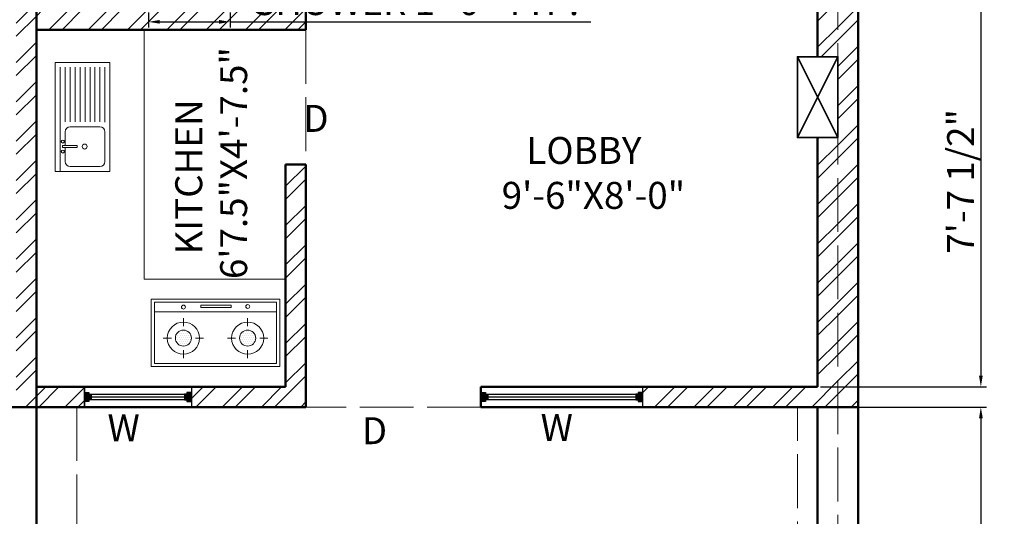
# Model space of a CAD drawing. Units: millimetres. Extents: x 4237 to 5109, y 21391 to 22486.
# Tile 10 of 17: x 4458 to 4678, y 22209 to 22320. Entities that reach past the tile are written whole.
import ezdxf

# ---------------------------------------------------------------- set-up
doc = ezdxf.new("R2010")
doc.units = ezdxf.units.MM
doc.linetypes.add('ACAD_ISO02W100', pattern=[15, 12, -3])
for name, color, linetype, lineweight in [('A-ANNO-DIMS', 2, 'Continuous', 18), ('A-ANNO-TEXT', 7, 'Continuous', 18), ('A-AREA-IDEN', 3, 'Continuous', 18), ('A-FLOR-OVHD', 1, 'ACAD_ISO02W100', 18), ('A-FURN', 8, 'Continuous', 18), ('A-WALL', 7, 'Continuous', 50), ('A-WALL-PATT', 252, 'Continuous', 13), ('column', 102, 'Continuous', 35), ('windows', 140, 'Continuous', 25)]:
    doc.layers.add(name, color=color, linetype=linetype, lineweight=lineweight)
doc.styles.get("Standard").update_dxf_attribs({"font": 'arial.ttf'})
doc.dimstyles.new('ISO-25', dxfattribs={"dimtxt": 6, "dimasz": 2.5, "dimexe": 1.25, "dimexo": 0.625, "dimtad": 1, "dimdec": 1, "dimlunit": 4, "dimtxsty": 'Standard', "dimcen": 2.5, "dimadec": 0, "dimazin": 0, "dimtfac": 1, "dimtdec": 1, "dimtmove": 0, "dimatfit": 3, "dimfxl": 1, "dimarcsym": 0})

# ---------------------------------------------------------------- blocks, each defined once
blk = doc.blocks.new('A$C678C741B')
for p, q in [((720, 378), (0, 378)), ((0, 0), (0, 378)), ((702, 360), (18, 360)), ((18, 18), (18, 360)), ((277, 329.9), (277, 344.2)), ((277, 344.2), (448.4, 344.2)), ((448.4, 344.2), (448.4, 329.9)), ((702, 18), (702, 360)), ((720, 0), (720, 378)), ((702, 306), (18, 306)), ((448.4, 329.9), (277, 329.9)), ((180, 226.9), (180, 271.9)), ((540, 226.9), (540, 271.9)), ((138.6, 174.8), (138.6, 174.8)), ((144.2, 186.1), (144.2, 186.1)), ((149.8, 174.8), (149.8, 174.8)), ((155.5, 186.1), (155.5, 186.1)), ((161.1, 197.3), (161.1, 197.3)), ((161.1, 174.8), (161.1, 174.8)), ((166.7, 186.1), (166.7, 186.1)), ((172.3, 197.3), (172.3, 197.3)), ((172.3, 174.8), (172.3, 174.8)), ((178, 186.1), (178, 186.1)), ((183.6, 197.3), (183.6, 197.3)), ((183.6, 174.8), (183.6, 174.8)), ((189.2, 186.1), (189.2, 186.1)), ((194.8, 197.3), (194.8, 197.3)), ((194.8, 174.8), (194.8, 174.8)), ((200.5, 186.1), (200.5, 186.1)), ((206.1, 174.8), (206.1, 174.8)), ((211.7, 186.1), (211.7, 186.1)), ((217.3, 174.8), (217.3, 174.8)), ((498.6, 174.8), (498.6, 174.8)), ((504.2, 186.1), (504.2, 186.1)), ((509.8, 174.8), (509.8, 174.8)), ((515.5, 186.1), (515.5, 186.1)), ((521.1, 197.3), (521.1, 197.3)), ((521.1, 174.8), (521.1, 174.8)), ((526.7, 186.1), (526.7, 186.1)), ((532.3, 197.3), (532.3, 197.3)), ((532.3, 174.8), (532.3, 174.8)), ((538, 186.1), (538, 186.1)), ((543.6, 197.3), (543.6, 197.3)), ((543.6, 174.8), (543.6, 174.8)), ((549.2, 186.1), (549.2, 186.1)), ((554.8, 197.3), (554.8, 197.3)), ((554.8, 174.8), (554.8, 174.8)), ((560.5, 186.1), (560.5, 186.1)), ((566.1, 174.8), (566.1, 174.8)), ((571.7, 186.1), (571.7, 186.1)), ((577.3, 174.8), (577.3, 174.8)), ((112.5, 159.4), (67.5, 159.4)), ((138.6, 152.3), (138.6, 152.3)), ((144.2, 163.6), (144.2, 163.6)), ((144.2, 141.1), (144.2, 141.1)), ((149.8, 152.3), (149.8, 152.3)), ((149.8, 129.8), (149.8, 129.8)), ((155.5, 163.6), (155.5, 163.6)), ((155.5, 141.1), (155.5, 141.1)), ((161.1, 152.3), (161.1, 152.3)), ((161.1, 129.8), (161.1, 129.8)), ((166.7, 163.6), (166.7, 163.6)), ((166.7, 141.1), (166.7, 141.1)), ((166.7, 118.6), (166.7, 118.6)), ((172.3, 152.3), (172.3, 152.3)), ((172.3, 129.8), (172.3, 129.8)), ((178, 163.6), (178, 163.6)), ((178, 141.1), (178, 141.1)), ((178, 118.6), (178, 118.6)), ((183.6, 152.3), (183.6, 152.3)), ((183.6, 129.8), (183.6, 129.8)), ((189.2, 163.6), (189.2, 163.6)), ((189.2, 141.1), (189.2, 141.1)), ((189.2, 118.6), (189.2, 118.6)), ((194.8, 152.3), (194.8, 152.3)), ((194.8, 129.8), (194.8, 129.8)), ((200.5, 163.6), (200.5, 163.6)), ((200.5, 141.1), (200.5, 141.1)), ((206.1, 152.3), (206.1, 152.3)), ((206.1, 129.8), (206.1, 129.8)), ((211.7, 163.6), (211.7, 163.6)), ((211.7, 141.1), (211.7, 141.1)), ((217.3, 152.3), (217.3, 152.3)), ((223, 163.6), (223, 163.6)), ((292.5, 159.4), (247.5, 159.4)), ((472.5, 159.4), (427.5, 159.4)), ((498.6, 152.3), (498.6, 152.3)), ((504.2, 163.6), (504.2, 163.6)), ((504.2, 141.1), (504.2, 141.1)), ((509.8, 152.3), (509.8, 152.3)), ((509.8, 129.8), (509.8, 129.8)), ((515.5, 163.6), (515.5, 163.6)), ((515.5, 141.1), (515.5, 141.1)), ((521.1, 152.3), (521.1, 152.3)), ((521.1, 129.8), (521.1, 129.8)), ((526.7, 163.6), (526.7, 163.6)), ((526.7, 141.1), (526.7, 141.1)), ((526.7, 118.6), (526.7, 118.6)), ((532.3, 152.3), (532.3, 152.3)), ((532.3, 129.8), (532.3, 129.8)), ((538, 163.6), (538, 163.6)), ((538, 141.1), (538, 141.1)), ((538, 118.6), (538, 118.6)), ((543.6, 152.3), (543.6, 152.3)), ((543.6, 129.8), (543.6, 129.8)), ((549.2, 163.6), (549.2, 163.6)), ((549.2, 141.1), (549.2, 141.1)), ((549.2, 118.6), (549.2, 118.6)), ((554.8, 152.3), (554.8, 152.3)), ((554.8, 129.8), (554.8, 129.8)), ((560.5, 163.6), (560.5, 163.6)), ((560.5, 141.1), (560.5, 141.1)), ((566.1, 152.3), (566.1, 152.3)), ((566.1, 129.8), (566.1, 129.8)), ((571.7, 163.6), (571.7, 163.6)), ((571.7, 141.1), (571.7, 141.1)), ((577.3, 152.3), (577.3, 152.3)), ((583, 163.6), (583, 163.6)), ((652.5, 159.4), (607.5, 159.4)), ((180, 46.9), (180, 91.9)), ((540, 46.9), (540, 91.9)), ((720, 0), (0, 0)), ((702, 18), (18, 18))]:
    blk.add_line(p, q)
for centre, radius in [((180.2, 333.1), 10.8), ((540.5, 336.3), 10.8), ((180, 159.4), 90), ((540, 159.4), 90), ((180, 159.4), 45), ((540, 159.4), 45)]:
    blk.add_circle(centre, radius)
blk = doc.blocks.new('A$C634174F9')
for p, q in [((0, 0), (0, 550)), ((0, 550), (1100, 550)), ((0, 500), (1052.1, 500)), ((1100, 550), (1100, 0)), ((50, 100), (50, 400)), ((100, 450), (240.4, 450)), ((240.9, 479), (240.9, 328.2)), ((260.9, 479), (240.9, 479)), ((260.9, 479), (260.9, 328.2)), ((261, 450), (400, 450)), ((450, 100), (450, 400)), ((501, 450), (1052.1, 450)), ((501, 400), (1052.1, 400)), ((240.9, 328.2), (260.9, 328.2)), ((501, 350), (1052.1, 350)), ((501, 300), (1052.1, 300)), ((501, 250), (1052.1, 250)), ((501, 200), (1052.1, 200)), ((501, 150), (1052.1, 150)), ((501, 100), (1052.1, 100)), ((1100, 0), (0, 0)), ((400, 50), (100, 50)), ((1052.1, 50), (498.4, 50))]:
    blk.add_line(p, q)
for centre, radius in [((200.7, 474.1), 15.3), ((301.1, 474.1), 15.3), ((250.7, 254), 25)]:
    blk.add_circle(centre, radius)
for centre, start, end in [((100, 400), 90, 180), ((100, 400), 90, 180), ((400, 400), 0, 90), ((400, 400), 0, 90), ((100, 100), 180, 270), ((400, 100), 270, 0)]:
    blk.add_arc(centre, 50, start, end)
blk = doc.blocks.new('WIN-A')
blk.add_line((0, 4.5), (0, 0))
blk.add_lwpolyline([(0, 4.5), (23.8, 4.5), (23.8, 0), (0, 0)], close=True)
blk = doc.blocks.new('*D90')
at = {"layer": 'A-ANNO-DIMS', "color": 0, "lineweight": -2, "transparency": 16777216}
for p, q in [((4486.92, 22321.58), (4486.92, 22318.22)), ((4505.11, 22321.58), (4505.11, 22318.22)), ((4489.42, 22319.47), (4502.61, 22319.47)), ((4505.11, 22319.47), (4585.45, 22319.47))]:
    blk.add_line(p, q, dxfattribs=at)
at = {"layer": 'A-ANNO-DIMS', "color": 0, "transparency": 16777216}
for points in [[(4489.42, 22319.89), (4489.42, 22319.06), (4486.92, 22319.47)], [(4502.61, 22319.89), (4502.61, 22319.06), (4505.11, 22319.47)]]:
    blk.add_solid(points, dxfattribs=at)
at = {"layer": 'Defpoints', "color": 0, "transparency": 16777216}
for p in [(4486.92, 22322.2), (4505.11, 22322.2), (4505.11, 22319.47)]:
    blk.add_point(p, dxfattribs=at)
at = {"layer": 'A-ANNO-DIMS', "color": 0, "transparency": 16777216, "insert": (4546.53, 22323.2), "char_height": 6, "attachment_point": 5}
blk.add_mtext('SHOWER 1\'-6" TYP.', dxfattribs=at)
blk = doc.blocks.new('*D102')
at = {"layer": 'A-ANNO-DIMS', "color": 0, "lineweight": -2, "transparency": 16777216}
for p, q in [((4461.95, 22233.08), (4461.95, 21960.6)), ((4452.95, 22185.08), (4452.95, 21960.6)), ((4455.45, 21961.85), (4459.45, 21961.85)), ((4461.95, 21961.85), (4481.65, 21961.85))]:
    blk.add_line(p, q, dxfattribs=at)
at = {"layer": 'A-ANNO-DIMS', "color": 0, "transparency": 16777216}
for points in [[(4455.45, 21962.27), (4455.45, 21961.43), (4452.95, 21961.85)], [(4459.45, 21962.27), (4459.45, 21961.43), (4461.95, 21961.85)]]:
    blk.add_solid(points, dxfattribs=at)
at = {"layer": 'Defpoints', "color": 0, "transparency": 16777216}
for p in [(4461.95, 22233.7), (4452.95, 22185.7), (4461.95, 21961.85)]:
    blk.add_point(p, dxfattribs=at)
at = {"layer": 'A-ANNO-DIMS', "color": 0, "transparency": 16777216, "insert": (4473.05, 21965.54), "char_height": 6, "attachment_point": 5}
blk.add_mtext('0\'-9"', dxfattribs=at)
blk = doc.blocks.new('*D103')
at = {"layer": 'A-ANNO-DIMS', "color": 0, "lineweight": -2, "transparency": 16777216}
for p, q in [((4461.95, 22233.08), (4461.95, 21960.6)), ((4635.95, 22233.08), (4635.95, 21960.6)), ((4464.45, 21961.85), (4633.45, 21961.85))]:
    blk.add_line(p, q, dxfattribs=at)
at = {"layer": 'A-ANNO-DIMS', "color": 0, "transparency": 16777216}
for points in [[(4464.45, 21962.27), (4464.45, 21961.43), (4461.95, 21961.85)], [(4633.45, 21962.27), (4633.45, 21961.43), (4635.95, 21961.85)]]:
    blk.add_solid(points, dxfattribs=at)
at = {"layer": 'Defpoints', "color": 0, "transparency": 16777216}
for p in [(4461.95, 22233.7), (4635.95, 22233.7), (4635.95, 21961.85)]:
    blk.add_point(p, dxfattribs=at)
at = {"layer": 'A-ANNO-DIMS', "color": 0, "transparency": 16777216, "insert": (4548.95, 21965.54), "char_height": 6, "attachment_point": 5}
blk.add_mtext('14\'-6"', dxfattribs=at)
blk = doc.blocks.new('*D104')
at = {"layer": 'A-ANNO-DIMS', "color": 0, "lineweight": -2, "transparency": 16777216}
for p, q in [((4635.95, 22233.08), (4635.95, 21960.6)), ((4644.95, 22032.08), (4644.95, 21960.6)), ((4638.45, 21961.85), (4642.45, 21961.85)), ((4644.95, 21961.85), (4664.65, 21961.85))]:
    blk.add_line(p, q, dxfattribs=at)
at = {"layer": 'A-ANNO-DIMS', "color": 0, "transparency": 16777216}
for points in [[(4638.45, 21962.27), (4638.45, 21961.43), (4635.95, 21961.85)], [(4642.45, 21962.27), (4642.45, 21961.43), (4644.95, 21961.85)]]:
    blk.add_solid(points, dxfattribs=at)
at = {"layer": 'Defpoints', "color": 0, "transparency": 16777216}
for p in [(4635.95, 22233.7), (4644.95, 22032.7), (4644.95, 21961.85)]:
    blk.add_point(p, dxfattribs=at)
at = {"layer": 'A-ANNO-DIMS', "color": 0, "transparency": 16777216, "insert": (4656.05, 21965.54), "char_height": 6, "attachment_point": 5}
blk.add_mtext('0\'-9"', dxfattribs=at)
blk = doc.blocks.new('*D106')
at = {"layer": 'A-ANNO-DIMS', "color": 0, "lineweight": -2, "transparency": 16777216}
for p, q in [((4636.58, 22329.7), (4673.55, 22329.7)), ((4672.3, 22327.2), (4672.3, 22240.7)), ((4636.58, 22238.2), (4673.55, 22238.2))]:
    blk.add_line(p, q, dxfattribs=at)
at = {"layer": 'A-ANNO-DIMS', "color": 0, "transparency": 16777216}
for points in [[(4671.88, 22327.2), (4672.72, 22327.2), (4672.3, 22329.7)], [(4671.88, 22240.7), (4672.72, 22240.7), (4672.3, 22238.2)]]:
    blk.add_solid(points, dxfattribs=at)
at = {"layer": 'Defpoints', "color": 0, "transparency": 16777216}
for p in [(4635.95, 22329.7), (4635.95, 22238.2), (4672.3, 22238.2)]:
    blk.add_point(p, dxfattribs=at)
at = {"layer": 'A-ANNO-DIMS', "color": 0, "transparency": 16777216, "insert": (4668.57, 22283.95), "char_height": 6, "attachment_point": 5, "rotation": 90}
blk.add_mtext('7\'-7 1/2"', dxfattribs=at)
blk = doc.blocks.new('*D107')
at = {"layer": 'A-ANNO-DIMS', "color": 0, "lineweight": -2, "transparency": 16777216}
for p, q in [((4636.58, 22233.7), (4673.55, 22233.7)), ((4672.3, 22231.2), (4672.3, 22035.2)), ((4645.58, 22032.7), (4673.55, 22032.7))]:
    blk.add_line(p, q, dxfattribs=at)
at = {"layer": 'A-ANNO-DIMS', "color": 0, "transparency": 16777216}
for points in [[(4671.88, 22231.2), (4672.72, 22231.2), (4672.3, 22233.7)], [(4671.88, 22035.2), (4672.72, 22035.2), (4672.3, 22032.7)]]:
    blk.add_solid(points, dxfattribs=at)
at = {"layer": 'Defpoints', "color": 0, "transparency": 16777216}
for p in [(4635.95, 22233.7), (4644.95, 22032.7), (4672.3, 22032.7)]:
    blk.add_point(p, dxfattribs=at)
at = {"layer": 'A-ANNO-DIMS', "color": 0, "transparency": 16777216, "insert": (4668.61, 22133.2), "char_height": 6, "attachment_point": 5, "rotation": 90}
blk.add_mtext('16\'-9"', dxfattribs=at)

msp = doc.modelspace()

# ---------------------------------------------------------------- hatches: boundary and pattern name
at = {"layer": 'A-WALL-PATT'}
h = msp.add_hatch(dxfattribs=at)
h.set_pattern_fill('ANSI32', color=256, scale=0.65)
h.paths.add_polyline_path([(4644.95, 22440.7), (4517.45, 22440.7), (4517.45, 22436.2), (4622.45, 22436.2), (4640.45, 22436.2), (4640.45, 22427.2), (4640.45, 22233.7), (4644.95, 22233.7)])
h = msp.add_hatch(dxfattribs=at)
h.set_pattern_fill('ANSI32', color=256, scale=0.65)
h.paths.add_polyline_path([(4640.45, 22427.2), (4635.95, 22427.2), (4635.95, 22334.2), (4560.95, 22334.2), (4560.95, 22332.95), (4561.95, 22332.95), (4561.95, 22332.56), (4562.47, 22332.56), (4562.47, 22331.34), (4561.95, 22331.34), (4561.95, 22330.95), (4560.95, 22330.95), (4560.95, 22329.7), (4635.95, 22329.7), (4635.95, 22311.7), (4640.45, 22311.7)], flags=17)
h = msp.add_hatch(dxfattribs=at)
h.set_pattern_fill('ANSI32', color=256, scale=0.65)
h.paths.add_polyline_path([(4461.95, 22415.2), (4457.45, 22415.2), (4457.45, 22233.7), (4461.95, 22233.7)])
h = msp.add_hatch(dxfattribs=at)
h.set_pattern_fill('ANSI32', color=256, scale=0.65)
h.paths.add_polyline_path([(4521.95, 22340.2), (4517.45, 22340.2), (4517.45, 22322.2), (4461.95, 22322.2), (4461.95, 22317.7), (4521.95, 22317.7)])
h = msp.add_hatch(dxfattribs=at)
h.set_pattern_fill('ANSI32', color=256, scale=0.65)
h.paths.add_polyline_path([(4640.45, 22293.7), (4635.95, 22293.7), (4635.95, 22238.2), (4596.95, 22238.2), (4596.95, 22233.7), (4640.45, 22233.7)], flags=17)
h = msp.add_hatch(dxfattribs=at)
h.set_pattern_fill('ANSI32', color=256, scale=0.65)
h.paths.add_polyline_path([(4521.95, 22287.7), (4517.45, 22287.7), (4517.45, 22238.2), (4496.45, 22238.2), (4496.45, 22233.7), (4521.95, 22233.7)])
h = msp.add_hatch(dxfattribs=at)
h.set_pattern_fill('ANSI32', color=256, scale=0.65)
h.paths.add_polyline_path([(4472.65, 22238.2), (4461.95, 22238.2), (4461.95, 22233.7), (4472.65, 22233.7)])
h = msp.add_hatch(color=256, dxfattribs=at)
h.dxf.hatch_style = 1
h.paths.add_polyline_path([(4474.17, 22236.56), (4473.65, 22236.56), (4473.65, 22236.95), (4472.65, 22236.95), (4472.65, 22234.95), (4473.65, 22234.95), (4473.65, 22235.34), (4474.17, 22235.34)])
h = msp.add_hatch(color=256, dxfattribs=at)
h.dxf.hatch_style = 1
h.paths.add_polyline_path([(4496.45, 22236.95), (4495.45, 22236.95), (4495.45, 22236.56), (4494.94, 22236.56), (4494.94, 22235.34), (4495.45, 22235.34), (4495.45, 22234.95), (4496.45, 22234.95)])
h = msp.add_hatch(color=256, dxfattribs=at)
h.dxf.hatch_style = 1
h.paths.add_polyline_path([(4562.47, 22236.56), (4561.95, 22236.56), (4561.95, 22236.95), (4560.95, 22236.95), (4560.95, 22234.95), (4561.95, 22234.95), (4561.95, 22235.34), (4562.47, 22235.34)])
h = msp.add_hatch(color=256, dxfattribs=at)
h.dxf.hatch_style = 1
h.paths.add_polyline_path([(4596.95, 22236.95), (4595.95, 22236.95), (4595.95, 22236.56), (4595.44, 22236.56), (4595.44, 22235.34), (4595.95, 22235.34), (4595.95, 22234.95), (4596.95, 22234.95)])

# ---------------------------------------------------------------- linework, layer by layer
at = {"layer": 'A-FLOR-OVHD'}
for p, q in [((4521.95, 22317.7), (4521.95, 22287.7)), ((4560.95, 22233.7), (4521.95, 22233.7))]:
    msp.add_line(p, q, dxfattribs=at)
for points in [[(4640.45, 22032.7), (4640.45, 22436.2), (4276.15, 22436.2), (4276.15, 22032.7)], [(4470.95, 22233.7), (4470.95, 22151.2), (4631.45, 22151.2), (4631.45, 22233.7)]]:
    msp.add_lwpolyline(points, dxfattribs=at)
at = {"layer": 'A-FURN'}
msp.add_lwpolyline([(4485.95, 22317.7), (4485.95, 22262.2), (4517.45, 22262.2)], dxfattribs=at)
at = {"layer": 'A-WALL'}
for p, q in [((4644.95, 22440.7), (4644.95, 22032.7)), ((4461.95, 22415.2), (4461.95, 22233.7)), ((4521.95, 22340.2), (4521.95, 22317.7)), ((4635.95, 22329.7), (4635.95, 22311.7)), ((4461.95, 22317.7), (4521.95, 22317.7)), ((4635.95, 22293.7), (4635.95, 22238.2)), ((4517.45, 22287.7), (4521.95, 22287.7)), ((4517.45, 22287.7), (4517.45, 22238.2)), ((4521.95, 22287.7), (4521.95, 22233.7)), ((4461.95, 22238.2), (4517.45, 22238.2)), ((4560.95, 22238.2), (4560.95, 22233.7)), ((4560.95, 22238.2), (4635.95, 22238.2)), ((4452.95, 22233.7), (4521.95, 22233.7)), ((4461.95, 22233.7), (4461.95, 22194.7)), ((4560.95, 22233.7), (4644.95, 22233.7)), ((4635.95, 22233.7), (4635.95, 22160.2))]:
    msp.add_line(p, q, dxfattribs=at)
at = {"layer": 'column'}
for p, q in [((4631.45, 22311.7), (4640.45, 22311.7)), ((4631.45, 22311.7), (4640.45, 22293.7)), ((4640.45, 22311.7), (4631.45, 22293.7)), ((4635.95, 22293.7), (4640.45, 22293.7))]:
    msp.add_line(p, q, dxfattribs=at)
msp.add_lwpolyline([(4640.45, 22293.7), (4631.45, 22293.7), (4631.45, 22311.7), (4640.45, 22311.7)], close=True, dxfattribs=at)
at = {"layer": 'windows'}
for p, q in [((4496.45, 22238.2), (4496.45, 22233.7)), ((4474.17, 22236.56), (4494.94, 22236.56)), ((4474.17, 22235.95), (4494.94, 22235.95)), ((4494.94, 22235.34), (4474.17, 22235.34)), ((4562.47, 22236.56), (4595.44, 22236.56)), ((4562.47, 22235.95), (4595.44, 22235.95)), ((4595.44, 22235.34), (4562.47, 22235.34))]:
    msp.add_line(p, q, dxfattribs=at)
msp.add_lwpolyline([(4560.95, 22238.2), (4596.95, 22238.2), (4596.95, 22233.7), (4560.95, 22233.7)], close=True, dxfattribs=at)
for points in [[(4472.65, 22236.95), (4473.65, 22236.95), (4473.65, 22236.56), (4474.17, 22236.56), (4474.17, 22235.34), (4473.65, 22235.34), (4473.65, 22234.95), (4472.65, 22234.95)], [(4496.45, 22236.95), (4495.45, 22236.95), (4495.45, 22236.56), (4494.94, 22236.56), (4494.94, 22235.34), (4495.45, 22235.34), (4495.45, 22234.95), (4496.45, 22234.95)], [(4560.95, 22236.95), (4561.95, 22236.95), (4561.95, 22236.56), (4562.47, 22236.56), (4562.47, 22235.34), (4561.95, 22235.34), (4561.95, 22234.95), (4560.95, 22234.95)], [(4596.95, 22236.95), (4595.95, 22236.95), (4595.95, 22236.56), (4595.44, 22236.56), (4595.44, 22235.34), (4595.95, 22235.34), (4595.95, 22234.95), (4596.95, 22234.95)]]:
    msp.add_lwpolyline(points, dxfattribs=at)

# ---------------------------------------------------------------- block references
at = {"layer": 'A-FURN', "xscale": 0.0220671414042477, "yscale": 0.0220671414042477, "zscale": 0.0220671414042477, "rotation": 90}
msp.add_blockref('A$C634174F9', (4478.29, 22286.17), dxfattribs=at)
at = {"layer": 'A-FURN', "xscale": 0.0397613605137319, "yscale": 0.0397613605137319, "zscale": 0.0397613605137319}
msp.add_blockref('A$C678C741B', (4487.52, 22242.72), dxfattribs=at)
at = {"layer": 'windows'}
msp.add_blockref('WIN-A', (4472.65, 22233.7), dxfattribs=at)

# ---------------------------------------------------------------- texts
at = {"layer": 'A-ANNO-TEXT', "char_height": 6, "attachment_point": 1}
for s, insert in [('    D', (4514.05, 22300.97)), ('    W', (4470.44, 22232.07)), ('    D', (4527.08, 22231.44)), ('    W', (4566.91, 22232.15))]:
    msp.add_mtext_dynamic_manual_height_columns(s, width=21.7253, gutter_width=12.5, heights=[0], dxfattribs=dict(at, insert=insert))
at = {"layer": 'A-AREA-IDEN', "insert": (4492.87, 22262.2), "char_height": 6, "attachment_point": 1, "rotation": 90}
msp.add_mtext_dynamic_manual_height_columns('   KITCHEN\\P6\'7.5"X4\'-7.5"', width=55.7646, gutter_width=12.5, heights=[0], dxfattribs=at)
at = {"layer": 'A-AREA-IDEN', "insert": (4563.74, 22293.84), "char_height": 6, "attachment_point": 1}
msp.add_mtext_dynamic_manual_height_columns('    LOBBY\\P 9\'-6"X8\'-0"', width=55.7646, gutter_width=12.5, heights=[0], dxfattribs=at)

# ---------------------------------------------------------------- dimensions: what is measured, and where the dimension line sits
at = {"layer": 'A-ANNO-DIMS'}
dim = msp.add_linear_dim(base=(4505.11, 22319.47), p1=(4486.92, 22322.2), p2=(4505.11, 22322.2), text='SHOWER <> TYP.', dimstyle='ISO-25', override={"dimdec": 1, "dimrnd": 0, "dimzin": 1, "dimlunit": 4, "dimfrac": 2}, dxfattribs=at)
dim.commit()
dim.dimension.update_dxf_attribs({"geometry": '*D90', "text_midpoint": (4546.53, 22323.2)})
for base, p1, p2, picture, middle in [((4672.3, 22238.2), (4635.95, 22329.7), (4635.95, 22238.2), '*D106', (4668.57, 22283.95)), ((4672.3, 22032.7), (4635.95, 22233.7), (4644.95, 22032.7), '*D107', (4668.61, 22133.2))]:
    dim = msp.add_linear_dim(base=base, p1=p1, p2=p2, angle=90, dimstyle='ISO-25', override={"dimdec": 1, "dimlfac": 1, "dimrnd": 0, "dimzin": 1, "dimdsep": 46, "dimlunit": 4, "dimfrac": 2}, dxfattribs=at)
    dim.commit()
    dim.dimension.update_dxf_attribs({"geometry": picture, "text_midpoint": middle})
for base, p1, p2, picture, middle in [((4461.95, 21961.85), (4452.95, 22185.7), (4461.95, 22233.7), '*D102', (4473.05, 21965.54)), ((4635.95, 21961.85), (4461.95, 22233.7), (4635.95, 22233.7), '*D103', (4548.95, 21965.54)), ((4644.95, 21961.85), (4635.95, 22233.7), (4644.95, 22032.7), '*D104', (4656.05, 21965.54))]:
    dim = msp.add_linear_dim(base=base, p1=p1, p2=p2, dimstyle='ISO-25', override={"dimdec": 1, "dimlfac": 1, "dimrnd": 0, "dimzin": 1, "dimdsep": 46, "dimlunit": 4, "dimfrac": 2}, dxfattribs=at)
    dim.commit()
    dim.dimension.update_dxf_attribs({"geometry": picture, "text_midpoint": middle})

doc.saveas('drawing.dxf')
